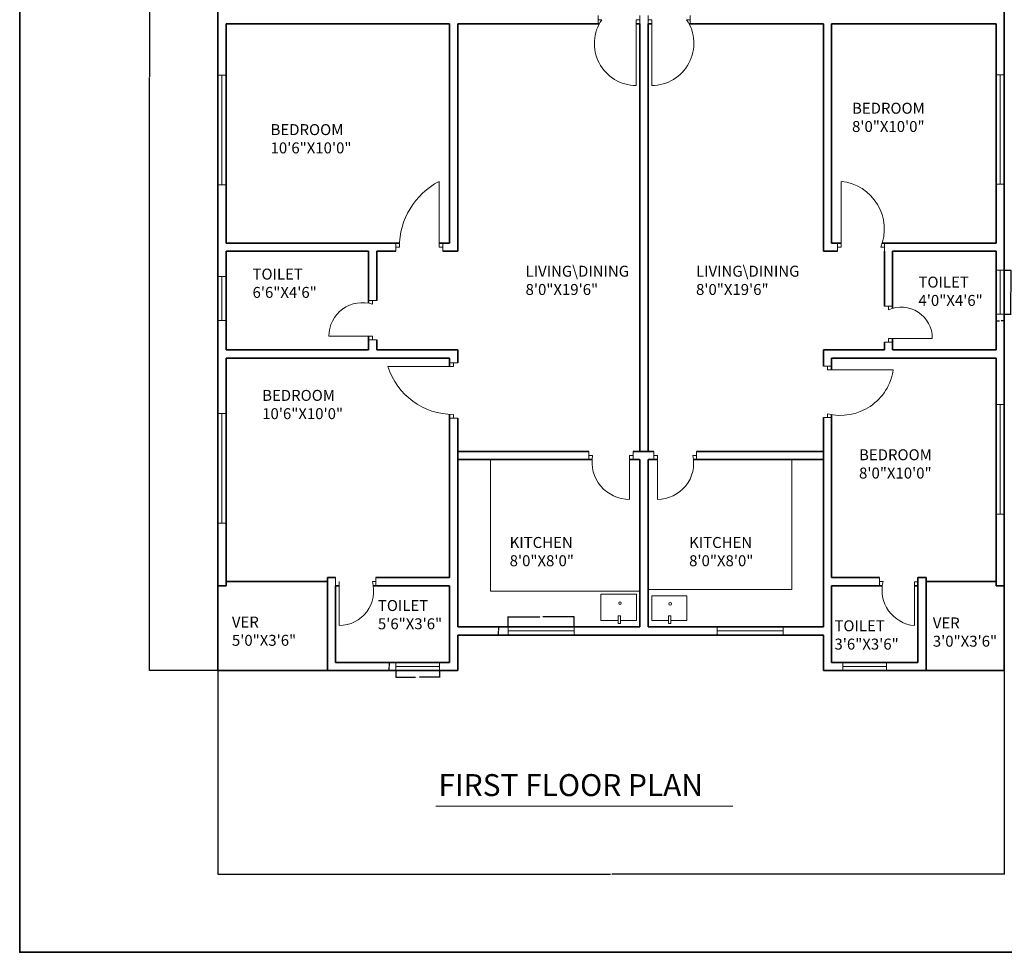
# Model space of a CAD drawing. Units: inches. Extents: x 992 to 2287, y 1476 to 2866.
# Tile 1 of 9: x 992 to 1531, y 1476 to 1987. Entities that reach past the tile are written whole.
import ezdxf

# ---------------------------------------------------------------- set-up
doc = ezdxf.new("R2010")
doc.units = ezdxf.units.IN
for name, color, linetype, lineweight in [('A-ANNO-DIMS', 2, 'Continuous', 18), ('A-ANNO-TEXT', 7, 'Continuous', 18), ('A-ANNO-TTLB', 7, 'Continuous', 35), ('A-AREA-IDEN', 7, 'Continuous', 18), ('A-DOOR', 3, 'Continuous', 18), ('A-FLOR-CASE', 9, 'Continuous', 18), ('A-FLOR-FIXT', 8, 'Continuous', 18), ('A-GLAZ', 4, 'Continuous', 18), ('A-WALL', 7, 'Continuous', 35)]:
    doc.layers.add(name, color=color, linetype=linetype, lineweight=lineweight)
doc.styles.get("Standard").update_dxf_attribs({"font": 'arial.ttf'})
doc.dimstyles.get("Standard").update_dxf_attribs({"dimtxt": 0.18, "dimasz": 0.18, "dimexe": 0.18, "dimexo": 0.0625, "dimgap": 0.09, "dimtad": 0, "dimtih": 1, "dimtoh": 1, "dimdec": 4, "dimzin": 0, "dimdsep": 46, "dimtxsty": 'Standard', "dimcen": 0.09, "dimadec": 0, "dimazin": 0, "dimtfac": 1, "dimtdec": 4, "dimtofl": 0, "dimtmove": 0, "dimatfit": 3, "dimfxl": 1, "dimtolj": 1, "dimtzin": 0, "dimarcsym": 0})

# ---------------------------------------------------------------- blocks, each defined once
blk = doc.blocks.new('DOOR-SINGLE-36IN-07')
for p, q in [((2.12, 38.25), (2.12, 33.75)), ((24.9, 33.75), (24.9, 38.25)), ((24.9, 38.25), (24.9, 36)), ((2.12, 36), (4.12, 36)), ((24.9, 36), (22.9, 36)), ((22.9, 36), (22.9, 0))]:
    blk.add_line(p, q)
blk.add_arc((22.9, 22.9), 22.9, 145.0915, 270)
blk = doc.blocks.new('DOOR-SINGLE-36IN-08')
for p, q in [((0, 33.75), (0, 38.25)), ((23.12, 38.25), (23.12, 33.75)), ((0, 36), (2, 36)), ((2, 36), (2, 0)), ((23.12, 36), (21.12, 36)), ((23.12, 33.75), (23.12, 36))]:
    blk.add_line(p, q)
blk.add_arc((2, 23.08), 23.08, 270, 34.0417)
blk = doc.blocks.new('DOOR-SINGLE-36IN-09')
for p, q in [((23.75, 2.25), (23.75, 38.25)), ((0, 4.5), (0, 0)), ((0, 0), (0, 2.25)), ((0, 2.25), (2, 2.25)), ((25.75, 2.25), (23.75, 2.25)), ((25.75, 4.5), (25.75, 0)), ((25.75, 0), (25.75, 2.25))]:
    blk.add_line(p, q)
blk.add_arc((42.67, 2.25), 40.67, 117.7196, 180)
blk = doc.blocks.new('DOOR-SINGLE-36IN-10')
for p, q in [((2, 2.25), (2, 38.25)), ((0, 4.5), (0, 0)), ((0, 0), (0, 2.25)), ((0, 2.25), (2, 2.25)), ((25.57, 2.25), (23.57, 2.25)), ((25.57, 0), (25.57, 4.5))]:
    blk.add_line(p, q)
blk.add_arc((-0.74, 12.15), 26.25, 337.8522, 84.002)
blk = doc.blocks.new('DOOR-SINGLE-24IN-11')
for p, q in [((21.75, 21.48), (26.25, 21.48)), ((26.25, 21.48), (24, 21.48)), ((24, 21.48), (24, 19.48)), ((24, 2), (0, 2)), ((26.25, 0), (21.75, 0)), ((21.75, 0), (24, 0)), ((24, 0), (24, 2))]:
    blk.add_line(p, q)
blk.add_arc((18.36, 2), 18.36, 72.1205, 180)
blk = doc.blocks.new('DOOR-SINGLE-24IN-12')
for p, q in [((0, 19.63), (4.5, 19.63)), ((4.5, 19.63), (2.25, 19.63)), ((2.25, 19.63), (2.25, 17.63)), ((2.25, 0), (2.25, 2)), ((2.25, 2), (26.25, 2)), ((4.5, 0), (0, 0)), ((0, 0), (2.25, 0))]:
    blk.add_line(p, q)
blk.add_arc((9.16, 2), 17.09, 0, 113.8439)
blk = doc.blocks.new('DOOR-SINGLE-24IN-13')
for p, q in [((0, 26.33), (0, 21.83)), ((0, 21.83), (0, 24.08)), ((0, 24.08), (2, 24.08)), ((21.14, 24), (19.14, 24)), ((19.14, 24), (19.14, 0))]:
    blk.add_line(p, q)
blk.add_arc((20.98, 19.45), 19.54, 166.3014, 264.5707)
blk = doc.blocks.new('DOOR-SINGLE-24IN-14')
for p, q in [((0, 21.75), (0, 26.25)), ((0, 26.25), (0, 24)), ((2, 24), (2, 0)), ((22.08, 24), (20.08, 24)), ((22.08, 26.25), (22.08, 21.75)), ((22.08, 21.75), (22.08, 24))]:
    blk.add_line(p, q)
blk.add_arc((2, 18.81), 18.81, 270, 16.0026)
blk = doc.blocks.new('DOOR-SINGLE-24IN-15')
for p, q in [((0, 26.25), (0, 21.75)), ((0, 21.75), (0, 24)), ((0, 24), (2, 24)), ((2, 24), (2, 0)), ((23.28, 24), (21.28, 24)), ((23.28, 26.25), (23.28, 21.75)), ((23.28, 21.75), (23.28, 24.87)), ((23.28, 24.87), (23.28, 24.87)), ((23.28, 24.87), (23.28, 24))]:
    blk.add_line(p, q)
blk.add_arc((2, 19.75), 19.75, 270, 12.442)
blk = doc.blocks.new('DOOR-SINGLE-24IN-16')
for p, q in [((0, 26.25), (0, 21.75)), ((0, 21.75), (0, 24)), ((0, 24), (2, 24)), ((24.23, 24), (22.23, 24)), ((22.23, 24), (22.23, 0)), ((24.23, 21.75), (24.23, 26.25)), ((24.23, 26.25), (24.23, 24))]:
    blk.add_line(p, q)
blk.add_arc((22.23, 20.52), 20.52, 170.2522, 270)
blk = doc.blocks.new('DOOR-SINGLE-36IN-17')
for p, q in [((36, 28.21), (0, 28.21)), ((38.25, 30.21), (33.75, 30.21)), ((33.75, 30.21), (33.75, 30.21)), ((33.75, 30.21), (36, 30.21)), ((36, 30.21), (36, 28.21)), ((33.75, 0), (33.75, 0)), ((33.75, 0), (38.25, 0)), ((36, 0), (36, 2)), ((38.25, 0), (36, 0))]:
    blk.add_line(p, q)
blk.add_arc((36, 39.83), 37.83, 197.8869, 270)
blk = doc.blocks.new('DOOR-SINGLE-36IN-18')
for p, q in [((4.5, 28.09), (0, 28.09)), ((0, 28.09), (2.25, 28.09)), ((2.25, 28.09), (2.25, 26.09)), ((2.25, 26.09), (38.25, 26.09)), ((4.5, 0), (0, 0)), ((0, 0), (2.25, 0)), ((2.25, 0), (2.25, 2))]:
    blk.add_line(p, q)
blk.add_arc((9.28, 30.44), 29.3, 256.1264, 351.459)
blk = doc.blocks.new('WINDOW-24IN-A')
for p, q in [((0, 24), (4.5, 24)), ((4.5, 24), (2.25, 24)), ((2.25, 24), (2.25, 0)), ((2.25, 0), (0, 0)), ((0, 0), (4.5, 0))]:
    blk.add_line(p, q)
blk = doc.blocks.new('WINDOW-60IN-A')
for p, q in [((4.5, 60), (0, 60)), ((0, 60), (2.25, 60)), ((2.25, 60), (2.25, 0)), ((2.25, 0), (0, 0)), ((0, 0), (4.5, 0))]:
    blk.add_line(p, q)
blk = doc.blocks.new('WINDOW-60IN-B')
for p, q in [((0, 4.5), (0, 0)), ((0, 0), (0, 2.25)), ((0, 2.25), (60, 2.25)), ((60, 2.25), (60, 4.5)), ((60, 4.5), (60, 0))]:
    blk.add_line(p, q)
blk = doc.blocks.new('WINDOW-36IN')
for p, q in [((0, 4.5), (0, 0)), ((0, 0), (0, 2.25)), ((0, 2.25), (36, 2.25)), ((36, 2.25), (36, 4.5)), ((36, 4.5), (36, 0))]:
    blk.add_line(p, q)
blk = doc.blocks.new('WINDOW-24IN-C')
for p, q in [((0, 24), (4.5, 24)), ((4.5, 24), (2.25, 24)), ((2.25, 24), (2.25, 0)), ((4.5, 0), (0, 0)), ((2.25, 0), (4.5, 0))]:
    blk.add_line(p, q)
blk = doc.blocks.new('COUNTER-L-SOUTHWEST')
for p, q in [((0, 72.06), (0, 0)), ((0, 0), (81.77, 0)), ((81.77, 0), (81.77, 0))]:
    blk.add_line(p, q)
blk = doc.blocks.new('COUNTER-L-SOUTHEAST')
for p, q in [((78.66, 0), (78.66, 71.1)), ((0, 0), (78.66, 0))]:
    blk.add_line(p, q)
blk = doc.blocks.new('*D39')
at = {"layer": 'A-ANNO-DIMS', "color": 0, "lineweight": -2, "transparency": 16777216}
for p, q in [((1198.15, 1630.48), (1198.15, 1626.76)), ((1222.15, 1630.48), (1222.15, 1626.76)), ((1198.33, 1626.94), (1209.04, 1626.94)), ((1221.97, 1626.94), (1211.27, 1626.94))]:
    blk.add_line(p, q, dxfattribs=at)
at = {"layer": 'A-ANNO-DIMS', "color": 0, "transparency": 16777216}
for points in [[(1198.33, 1626.97), (1198.33, 1626.91), (1198.15, 1626.94)], [(1221.97, 1626.97), (1221.97, 1626.91), (1222.15, 1626.94)]]:
    blk.add_solid(points, dxfattribs=at)
at = {"layer": 'Defpoints', "color": 0, "transparency": 16777216}
for p in [(1198.15, 1630.54), (1222.15, 1630.54), (1198.15, 1626.94)]:
    blk.add_point(p, dxfattribs=at)
at = {"layer": 'A-ANNO-DIMS', "color": 0, "transparency": 16777216, "insert": (1210.15, 1626.94), "char_height": 0.18, "attachment_point": 5}
blk.add_mtext('\\A1;WINDOW 24 TYP.', dxfattribs=at)
blk = doc.blocks.new('*D40')
at = {"layer": 'A-ANNO-DIMS', "color": 0, "lineweight": -2, "transparency": 16777216}
for p, q in [((1198.09, 1635.04), (1194.37, 1635.04)), ((1194.55, 1634.86), (1194.55, 1632.97)), ((1198.09, 1630.54), (1194.37, 1630.54)), ((1194.55, 1630.72), (1194.55, 1632.61))]:
    blk.add_line(p, q, dxfattribs=at)
at = {"layer": 'A-ANNO-DIMS', "color": 0, "transparency": 16777216}
for points in [[(1194.52, 1634.86), (1194.58, 1634.86), (1194.55, 1635.04)], [(1194.52, 1630.72), (1194.58, 1630.72), (1194.55, 1630.54)]]:
    blk.add_solid(points, dxfattribs=at)
at = {"layer": 'Defpoints', "color": 0, "transparency": 16777216}
for p in [(1194.55, 1635.04), (1198.15, 1635.04), (1198.15, 1630.54)]:
    blk.add_point(p, dxfattribs=at)
at = {"layer": 'A-ANNO-DIMS', "color": 0, "transparency": 16777216, "insert": (1194.55, 1632.79), "char_height": 0.18, "attachment_point": 5}
blk.add_mtext('\\A1;5 TYP.', dxfattribs=at)
blk = doc.blocks.new('*D43')
at = {"layer": 'A-ANNO-DIMS', "color": 0, "lineweight": -2, "transparency": 16777216}
for p, q in [((1259.8, 1654.61), (1259.8, 1660.12)), ((1295.8, 1654.61), (1295.8, 1660.12)), ((1259.98, 1659.94), (1276.99, 1659.94)), ((1295.62, 1659.94), (1278.61, 1659.94))]:
    blk.add_line(p, q, dxfattribs=at)
at = {"layer": 'A-ANNO-DIMS', "color": 0, "transparency": 16777216}
for points in [[(1259.98, 1659.97), (1259.98, 1659.91), (1259.8, 1659.94)], [(1295.62, 1659.97), (1295.62, 1659.91), (1295.8, 1659.94)]]:
    blk.add_solid(points, dxfattribs=at)
at = {"layer": 'Defpoints', "color": 0, "transparency": 16777216}
for p in [(1295.8, 1659.94), (1259.8, 1654.54), (1295.8, 1654.54)]:
    blk.add_point(p, dxfattribs=at)
at = {"layer": 'A-ANNO-DIMS', "color": 0, "transparency": 16777216, "insert": (1277.8, 1659.94), "char_height": 0.18, "attachment_point": 5}
blk.add_mtext('\\A1;WIN 36 TYP.', dxfattribs=at)
blk = doc.blocks.new('*D44')
at = {"layer": 'A-ANNO-DIMS', "color": 0, "lineweight": -2, "transparency": 16777216}
for p, q in [((1259.74, 1654.54), (1254.22, 1654.54)), ((1259.74, 1650.04), (1254.22, 1650.04)), ((1254.4, 1654.36), (1254.4, 1652.47)), ((1254.4, 1650.22), (1254.4, 1652.11))]:
    blk.add_line(p, q, dxfattribs=at)
at = {"layer": 'A-ANNO-DIMS', "color": 0, "transparency": 16777216}
for points in [[(1254.37, 1654.36), (1254.43, 1654.36), (1254.4, 1654.54)], [(1254.37, 1650.22), (1254.43, 1650.22), (1254.4, 1650.04)]]:
    blk.add_solid(points, dxfattribs=at)
at = {"layer": 'Defpoints', "color": 0, "transparency": 16777216}
for p in [(1254.4, 1654.54), (1259.8, 1654.54), (1259.8, 1650.04)]:
    blk.add_point(p, dxfattribs=at)
at = {"layer": 'A-ANNO-DIMS', "color": 0, "transparency": 16777216, "insert": (1254.4, 1652.29), "char_height": 0.18, "attachment_point": 5}
blk.add_mtext('\\A1;5 TYP.', dxfattribs=at)
blk = doc.blocks.new('*D45')
at = {"layer": 'A-ANNO-DIMS', "color": 0, "lineweight": -2, "transparency": 16777216}
for p, q in [((1531.36, 1849.65), (1535.07, 1849.65)), ((1534.89, 1849.47), (1534.89, 1837.83)), ((1534.89, 1825.83), (1534.89, 1837.47)), ((1531.36, 1825.65), (1535.07, 1825.65))]:
    blk.add_line(p, q, dxfattribs=at)
at = {"layer": 'A-ANNO-DIMS', "color": 0, "transparency": 16777216}
for points in [[(1534.86, 1849.47), (1534.92, 1849.47), (1534.89, 1849.65)], [(1534.86, 1825.83), (1534.92, 1825.83), (1534.89, 1825.65)]]:
    blk.add_solid(points, dxfattribs=at)
at = {"layer": 'Defpoints', "color": 0, "transparency": 16777216}
for p in [(1531.29, 1849.65), (1534.89, 1849.65), (1531.29, 1825.65)]:
    blk.add_point(p, dxfattribs=at)
at = {"layer": 'A-ANNO-DIMS', "color": 0, "transparency": 16777216, "insert": (1534.89, 1837.65), "char_height": 0.18, "attachment_point": 5}
blk.add_mtext('\\A1;WINDOW 24 TYP.', dxfattribs=at)
blk = doc.blocks.new('*D46')
at = {"layer": 'A-ANNO-DIMS', "color": 0, "lineweight": -2, "transparency": 16777216}
for p, q in [((1526.79, 1825.59), (1526.79, 1821.87)), ((1526.97, 1822.05), (1528.59, 1822.05)), ((1531.11, 1822.05), (1529.5, 1822.05)), ((1531.29, 1825.59), (1531.29, 1821.87))]:
    blk.add_line(p, q, dxfattribs=at)
at = {"layer": 'A-ANNO-DIMS', "color": 0, "transparency": 16777216}
for points in [[(1526.97, 1822.08), (1526.97, 1822.02), (1526.79, 1822.05)], [(1531.11, 1822.08), (1531.11, 1822.02), (1531.29, 1822.05)]]:
    blk.add_solid(points, dxfattribs=at)
at = {"layer": 'Defpoints', "color": 0, "transparency": 16777216}
for p in [(1526.79, 1825.65), (1531.29, 1825.65), (1531.29, 1822.05)]:
    blk.add_point(p, dxfattribs=at)
at = {"layer": 'A-ANNO-DIMS', "color": 0, "transparency": 16777216, "insert": (1529.04, 1822.05), "char_height": 0.18, "attachment_point": 5}
blk.add_mtext('\\A1;5 TYP.', dxfattribs=at)
blk = doc.blocks.new('*D109')
at = {"layer": 'A-ANNO-DIMS', "color": 0, "lineweight": -2, "transparency": 16777216}
for p, q in [((1100.79, 1630.48), (1100.79, 1518.97)), ((1531.29, 1630.48), (1531.29, 1518.97)), ((1100.97, 1519.15), (1315.65, 1519.15)), ((1531.11, 1519.15), (1316.44, 1519.15))]:
    blk.add_line(p, q, dxfattribs=at)
at = {"layer": 'A-ANNO-DIMS', "color": 0, "transparency": 16777216}
for points in [[(1100.97, 1519.18), (1100.97, 1519.12), (1100.79, 1519.15)], [(1531.11, 1519.18), (1531.11, 1519.12), (1531.29, 1519.15)]]:
    blk.add_solid(points, dxfattribs=at)
at = {"layer": 'Defpoints', "color": 0, "transparency": 16777216}
for p in [(1100.79, 1630.54), (1531.29, 1630.54), (1531.29, 1519.15)]:
    blk.add_point(p, dxfattribs=at)
at = {"layer": 'A-ANNO-DIMS', "color": 0, "transparency": 16777216, "insert": (1316.04, 1519.15), "char_height": 0.18, "attachment_point": 5}
blk.add_mtext('\\A1;430.5', dxfattribs=at)
blk = doc.blocks.new('*D110')
at = {"layer": 'A-ANNO-DIMS', "color": 0, "lineweight": -2, "transparency": 16777216}
for p, q in [((1100.73, 2280.04), (1063.31, 2280.04)), ((1063.49, 2279.86), (1063.49, 1955.47)), ((1063.49, 1630.72), (1063.49, 1955.11)), ((1100.73, 1630.54), (1063.31, 1630.54))]:
    blk.add_line(p, q, dxfattribs=at)
at = {"layer": 'A-ANNO-DIMS', "color": 0, "transparency": 16777216}
for points in [[(1063.46, 2279.86), (1063.52, 2279.86), (1063.49, 2280.04)], [(1063.46, 1630.72), (1063.52, 1630.72), (1063.49, 1630.54)]]:
    blk.add_solid(points, dxfattribs=at)
at = {"layer": 'Defpoints', "color": 0, "transparency": 16777216}
for p in [(1063.49, 2280.04), (1100.79, 2280.04), (1100.79, 1630.54)]:
    blk.add_point(p, dxfattribs=at)
at = {"layer": 'A-ANNO-DIMS', "color": 0, "transparency": 16777216, "insert": (1063.49, 1955.29), "char_height": 0.18, "attachment_point": 5}
blk.add_mtext('\\A1;649.5', dxfattribs=at)

msp = doc.modelspace()

# ---------------------------------------------------------------- linework, layer by layer
at = {"layer": 'A-ANNO-TEXT'}
msp.add_line((1220.0701, 1556.4506), (1382.7129, 1556.4506), dxfattribs=at)
at = {"layer": 'A-ANNO-TTLB'}
msp.add_lwpolyline([(992.3484, 2866.1952), (2287.217, 2866.1952), (2287.217, 1476.4066), (992.3484, 1476.4066)], close=True, dxfattribs=at)
at = {"layer": 'A-FLOR-FIXT'}
for points in [[(1319.9654, 1657.9945), (1310.4914, 1657.9945), (1310.4914, 1672.436), (1330.0021, 1672.436), (1330.0021, 1657.9945), (1321.1582, 1657.9945)], [(1347.4819, 1657.9814), (1338.4372, 1657.9814), (1338.4372, 1671.5548), (1357.5926, 1671.5548), (1357.5926, 1657.9814), (1348.729, 1657.9814)]]:
    msp.add_lwpolyline(points, dxfattribs=at)
for points in [[(1319.9654, 1656.3749), (1321.1582, 1656.3749), (1321.1582, 1660.6263), (1319.9654, 1660.6263)], [(1347.4819, 1656.4254), (1348.729, 1656.4254), (1348.729, 1660.5731), (1347.4819, 1660.5731)]]:
    msp.add_lwpolyline(points, close=True, dxfattribs=at)
for centre, radius in [((1320.9331, 1667.4872), 0.7198), ((1348.4116, 1667.1007), 0.68)]:
    msp.add_circle(centre, radius, dxfattribs=at)
at = {"layer": 'A-WALL'}
for p, q in [((1100.7936, 2280.0428), (1100.7936, 1677.0428)), ((1531.2936, 2280.0428), (1531.2936, 1677.0428)), ((1531.2936, 1989.0428), (1531.2936, 1984.5428)), ((1105.2936, 1984.5428), (1227.5825, 1984.5428)), ((1105.2936, 1984.5428), (1105.2936, 1864.5428)), ((1227.5825, 1984.5428), (1227.5825, 1864.5428)), ((1232.0825, 1984.5428), (1232.0825, 1860.0428)), ((1232.0825, 1984.5428), (1303.2936, 1984.5428)), ((1309.6323, 1984.5428), (1303.2936, 1984.5428)), ((1331.7936, 1984.5428), (1329.7936, 1984.5428)), ((1331.7936, 1984.5428), (1331.7936, 1750.5428)), ((1336.2936, 1984.5428), (1336.2936, 1750.5428)), ((1338.2936, 1984.5428), (1336.2936, 1984.5428)), ((1432.2936, 1984.5428), (1358.759, 1984.5428)), ((1432.2936, 1984.5428), (1432.2936, 1860.0428)), ((1526.7936, 1984.5428), (1436.7936, 1984.5428)), ((1436.7936, 1984.5428), (1436.7936, 1864.5428)), ((1526.7936, 1984.5428), (1526.7936, 1864.5428)), ((1105.2936, 1864.5428), (1200.2142, 1864.5428)), ((1105.2936, 1860.0428), (1183.2936, 1860.0428)), ((1105.2936, 1860.0428), (1105.2936, 1806.0428)), ((1105.2936, 1860.0428), (1183.2936, 1860.0428)), ((1183.2936, 1860.0428), (1183.2936, 1831.6144)), ((1187.7936, 1860.0428), (1198.1519, 1860.0428)), ((1187.7936, 1833.0428), (1187.7936, 1860.0428)), ((1221.903, 1864.5428), (1227.5825, 1864.5428)), ((1223.903, 1860.0428), (1232.0825, 1860.0428)), ((1440.0708, 1860.0428), (1432.2936, 1860.0428)), ((1442.0708, 1864.5428), (1436.7936, 1864.5428)), ((1526.7936, 1864.5428), (1464.4381, 1864.5428)), ((1465.6395, 1830.0352), (1465.6395, 1860.0428)), ((1526.7936, 1860.0428), (1470.1395, 1860.0428)), ((1526.7936, 1860.0428), (1470.1395, 1860.0428)), ((1470.1395, 1860.0428), (1470.1395, 1828.8466)), ((1526.7936, 1860.0428), (1526.7936, 1806.0428)), ((1183.2936, 1813.5672), (1183.2936, 1806.0428)), ((1187.7936, 1806.0428), (1187.7936, 1811.5672)), ((1470.1395, 1812.4029), (1470.1395, 1806.0428)), ((1105.2936, 1806.0428), (1183.2936, 1806.0428)), ((1187.7936, 1806.0428), (1232.0825, 1806.0428)), ((1232.0825, 1806.0428), (1232.0825, 1798.922)), ((1432.2936, 1806.0428), (1432.2936, 1797.1964)), ((1465.6395, 1806.0428), (1432.2936, 1806.0428)), ((1465.6395, 1806.0428), (1465.6395, 1810.4029)), ((1526.7936, 1806.0428), (1470.1395, 1806.0428)), ((1105.2936, 1801.5428), (1227.5825, 1801.5428)), ((1105.2936, 1801.5428), (1105.2936, 1681.5428)), ((1227.5825, 1801.5428), (1227.5825, 1796.922)), ((1526.7936, 1801.5428), (1436.7936, 1801.5428)), ((1436.7936, 1801.5428), (1436.7936, 1795.1964)), ((1526.7936, 1801.5428), (1526.7936, 1681.5428)), ((1227.5825, 1770.7792), (1227.5825, 1681.5428)), ((1232.0825, 1768.7122), (1232.0825, 1654.5428)), ((1432.2936, 1769.1032), (1432.2936, 1654.5428)), ((1436.7936, 1770.6402), (1436.7936, 1681.5428)), ((1232.0825, 1750.5428), (1303.8904, 1750.5428)), ((1328.119, 1750.5428), (1339.497, 1750.5428)), ((1362.779, 1750.5428), (1432.2936, 1750.5428)), ((1232.0825, 1746.0428), (1305.6307, 1746.0428)), ((1326.119, 1746.0428), (1331.7936, 1746.0428)), ((1331.7936, 1746.0428), (1331.7936, 1654.5428)), ((1336.2936, 1746.0428), (1341.497, 1746.0428)), ((1336.2936, 1746.0428), (1336.2936, 1654.5428)), ((1361.1407, 1746.0428), (1432.2936, 1746.0428)), ((1105.2936, 1681.5428), (1105.2936, 1677.0428)), ((1160.7936, 1681.5428), (1165.2936, 1681.5428)), ((1160.7936, 1677.0428), (1160.7936, 1681.5428)), ((1187.378, 1681.5428), (1227.5825, 1681.5428)), ((1462.9081, 1681.5428), (1436.7936, 1681.5428)), ((1488.5436, 1681.5428), (1484.0436, 1681.5428)), ((1484.0436, 1681.5428), (1484.0436, 1635.0428)), ((1488.5436, 1635.0428), (1488.5436, 1681.5428)), ((1526.7936, 1681.5428), (1526.7936, 1677.0428)), ((1100.7936, 1677.0428), (1105.2936, 1677.0428)), ((1100.7936, 1677.0428), (1105.2936, 1677.0428)), ((1100.7936, 1677.0428), (1100.7936, 1630.5428)), ((1160.7936, 1679.2928), (1105.2936, 1679.2928)), ((1160.7936, 1677.0428), (1160.7936, 1630.5428)), ((1165.2936, 1635.0428), (1165.2936, 1677.0428)), ((1165.2936, 1677.0428), (1167.2936, 1677.0428)), ((1185.8764, 1677.0428), (1227.5825, 1677.0428)), ((1227.5825, 1677.0428), (1227.5825, 1635.0428)), ((1436.7936, 1677.0428), (1436.7936, 1635.0428)), ((1464.4975, 1677.0428), (1436.7936, 1677.0428)), ((1484.0436, 1677.0428), (1482.0436, 1677.0428)), ((1484.0436, 1677.0428), (1482.0436, 1677.0428)), ((1526.7936, 1679.2928), (1488.5436, 1679.2928)), ((1531.2936, 1677.0428), (1526.7936, 1677.0428)), ((1531.2936, 1677.0428), (1531.2936, 1631.5386)), ((1232.0825, 1654.5428), (1331.7936, 1654.5428)), ((1232.0825, 1650.0428), (1432.2936, 1650.0428)), ((1232.0825, 1650.0428), (1232.0825, 1630.5428)), ((1336.2936, 1654.5428), (1432.2936, 1654.5428)), ((1432.2936, 1650.0428), (1432.2936, 1630.5428)), ((1165.2936, 1635.0428), (1227.5825, 1635.0428)), ((1436.7936, 1635.0428), (1484.0436, 1635.0428)), ((1488.5436, 1635.0428), (1488.5436, 1630.5428)), ((1100.7936, 1630.5428), (1232.0825, 1630.5428)), ((1432.2936, 1630.5428), (1531.2936, 1630.5428)), ((1531.2936, 1631.5386), (1531.2936, 1630.5428))]:
    msp.add_line(p, q, dxfattribs=at)

# ---------------------------------------------------------------- block references
at = {"layer": 'A-DOOR'}
for name, p in [('DOOR-SINGLE-36IN-07', (1306.897, 1950.793)), ('DOOR-SINGLE-36IN-08', (1336.294, 1950.793)), ('DOOR-SINGLE-36IN-09', (1198.152, 1860.043)), ('DOOR-SINGLE-36IN-10', (1440.071, 1860.043)), ('DOOR-SINGLE-24IN-11', (1161.544, 1811.567)), ('DOOR-SINGLE-24IN-12', (1465.64, 1810.403)), ('DOOR-SINGLE-36IN-17', (1193.832, 1768.712)), ('DOOR-SINGLE-36IN-18', (1432.294, 1769.103)), ('DOOR-SINGLE-24IN-16', (1303.89, 1724.293)), ('DOOR-SINGLE-24IN-15', (1339.497, 1724.293)), ('DOOR-SINGLE-24IN-14', (1165.294, 1655.293)), ('DOOR-SINGLE-24IN-13', (1462.908, 1655.213))]:
    msp.add_blockref(name, p, dxfattribs=at)
at = {"layer": 'A-FLOR-CASE'}
for name, p in [('COUNTER-L-SOUTHWEST', (1250.019, 1673.984)), ('COUNTER-L-SOUTHEAST', (1336.294, 1674.941))]:
    msp.add_blockref(name, p, dxfattribs=at)
at = {"layer": 'A-GLAZ'}
for name, p in [('WINDOW-60IN-A', (1100.794, 1896.4076)), ('WINDOW-24IN-C', (1526.794, 1825.649)), ('WINDOW-36IN', (1259.803, 1650.043))]:
    msp.add_blockref(name, p, dxfattribs=at)
for name, p, rotation in [('WINDOW-60IN-B', (1531.2933, 1896.7008), 90), ('WINDOW-24IN-C', (1105.2931, 1846.2116), 180), ('WINDOW-60IN-B', (1531.2933, 1716.1491), 90), ('WINDOW-24IN-A', (1222.1538, 1630.5432), 90)]:
    msp.add_blockref(name, p, dxfattribs=dict(at, rotation=rotation))
at = {"layer": 'A-GLAZ', "extrusion": (0, 0, -1), "zscale": -1}
for name, p, rotation in [('WINDOW-60IN-B', (-1100.7938, 1711.2492), 90), ('WINDOW-36IN', (-1374.1934, 1654.5426), 180), ('WINDOW-24IN-A', (-1442.8595, 1630.5432), 90)]:
    msp.add_blockref(name, p, dxfattribs=dict(at, rotation=rotation))

# ---------------------------------------------------------------- texts
at = {"layer": 'A-ANNO-TEXT', "insert": (1221.559, 1573.916), "char_height": 12, "attachment_point": 1}
msp.add_mtext_dynamic_manual_height_columns('FIRST FLOOR PLAN', width=414.360918, gutter_width=12.5, heights=[0], dxfattribs=at)
at = {"layer": 'A-AREA-IDEN', "char_height": 6, "attachment_point": 1}
for s, width, insert in [('BEDROOM\\P8\'0"X10\'0"', 81.09558, (1447.948, 1941.3467)), ('BEDROOM\\P10\'6"X10\'0"', 166.036551, (1129.6941, 1929.6309)), ('TOILET\\P6\'6"X4\'6"', 103.27962, (1119.7942, 1850.5717)), ('LIVING\\\\DINING\\P8\'0"X19\'6"', 86.350152, (1269.2529, 1852.1494)), ('LIVING\\\\DINING\\P8\'0"X19\'6"', 86.350152, (1362.5508, 1852.1494)), ('TOILET\\P4\'0"X4\'6"', 46.991583, (1484.302, 1846.1707)), ('BEDROOM\\P10\'6"X10\'0"', 188.267406, (1125.0877, 1784.1907)), ('BEDROOM\\P8\'0"X10\'0"', 79.504257, (1451.7893, 1751.6873)), ('KITCHEN\\P8\'0"X8\'0"', 64.067345, (1260.5348, 1703.7017)), ('KITCHEN\\P8\'0"X8\'0"', 87.367603, (1358.7701, 1703.6897)), ('TOILET\\P5\'6"X3\'6"', 64.635723, (1188.4132, 1669.1933)), ('VER\\P5\'0"X3\'6"', 46.339212, (1108.5036, 1660.1438)), ('TOILET\\P3\'6"X3\'6"', 64.635723, (1438.3192, 1658.0867)), ('VER\\P3\'0"X3\'6"', 45.363663, (1492.1679, 1659.6703))]:
    msp.add_mtext_dynamic_manual_height_columns(s, width=width, gutter_width=12.5, heights=[0], dxfattribs=dict(at, insert=insert))

# ---------------------------------------------------------------- dimensions: what is measured, and where the dimension line sits
at = {"layer": 'A-ANNO-DIMS'}
dim = msp.add_linear_dim(base=(1063.4936, 2280.0428), p1=(1100.7936, 1630.5428), p2=(1100.7936, 2280.0428), angle=90, dimstyle='Standard', override={"dimdec": 1, "dimlfac": 1, "dimrnd": 0, "dimzin": 0, "dimdsep": 46, "dimlunit": 2}, dxfattribs=at)
dim.commit()
dim.dimension.update_dxf_attribs({"geometry": '*D110', "text_midpoint": (1063.4936, 1955.2928)})
for base, p1, p2, angle, text, picture, middle in [((1534.8936, 1849.6487), (1531.2936, 1825.6487), (1531.2936, 1849.6487), 90, 'WINDOW <> TYP.', '*D45', (1534.8936, 1837.6487)), ((1254.4028025431, 1654.542787875), (1259.8028025431, 1650.042787875), (1259.8028025431, 1654.542787875), 90, '<> TYP.', '*D44', (1254.4028025431, 1652.292787875)), ((1194.554072937, 1635.042787875), (1198.154072937, 1630.542787875), (1198.154072937, 1635.042787875), 90, '<> TYP.', '*D40', (1194.554072937, 1632.792787875)), ((1198.1541, 1626.9428), (1222.1541, 1630.5428), (1198.1541, 1630.5428), 180, 'WINDOW <> TYP.', '*D39', (1210.1541, 1626.9428))]:
    dim = msp.add_linear_dim(base=base, p1=p1, p2=p2, angle=angle, text=text, dimstyle='Standard', override={"dimdec": 0, "dimlfac": 1, "dimrnd": 0, "dimzin": 0, "dimdsep": 46, "dimlunit": 2}, dxfattribs=at)
    dim.commit()
    dim.dimension.update_dxf_attribs({"geometry": picture, "text_midpoint": middle})
for base, p1, p2, text, picture, middle in [((1531.2935507769, 1822.0487024318), (1526.7935507769, 1825.6487024318), (1531.2935507769, 1825.6487024318), '<> TYP.', '*D46', (1529.0435507769, 1822.0487024318)), ((1295.8028, 1659.9428), (1259.8028, 1654.5428), (1295.8028, 1654.5428), 'WIN <> TYP.', '*D43', (1277.8028, 1659.9428))]:
    dim = msp.add_linear_dim(base=base, p1=p1, p2=p2, text=text, dimstyle='Standard', override={"dimdec": 0, "dimlfac": 1, "dimrnd": 0, "dimzin": 0, "dimdsep": 46, "dimlunit": 2}, dxfattribs=at)
    dim.commit()
    dim.dimension.update_dxf_attribs({"geometry": picture, "text_midpoint": middle})
dim = msp.add_linear_dim(base=(1531.2936, 1519.1506), p1=(1100.7936, 1630.5428), p2=(1531.2936, 1630.5428), dimstyle='Standard', override={"dimdec": 1, "dimlfac": 1, "dimrnd": 0, "dimzin": 0, "dimdsep": 46, "dimlunit": 2}, dxfattribs=at)
dim.commit()
dim.dimension.update_dxf_attribs({"geometry": '*D109', "text_midpoint": (1316.0436, 1519.1506)})

doc.saveas('drawing.dxf')
